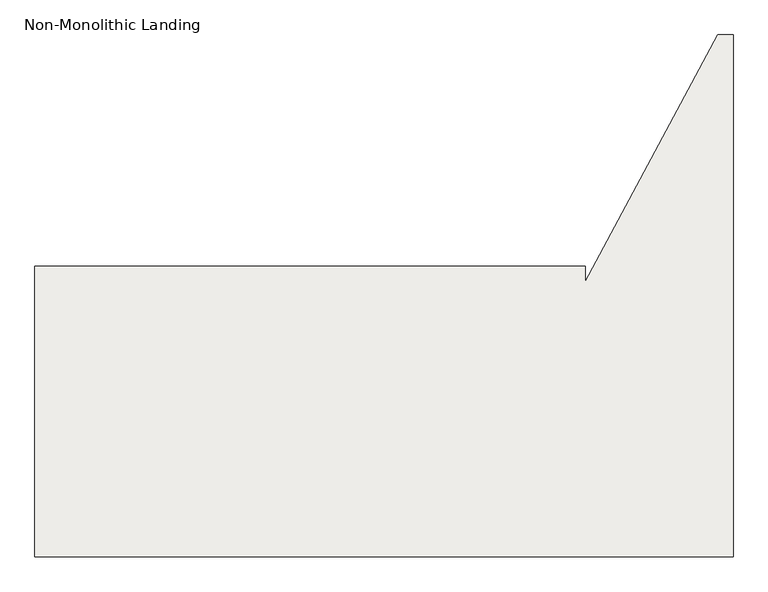
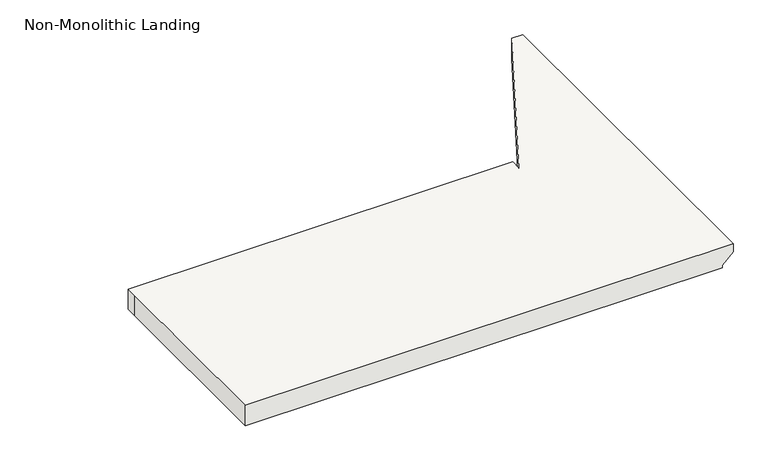
"""IFC4 building model written with IfcOpenShell, lengths in millimetres: slab geometry, Non-Monolithic Landing."""

from ifc_helpers import new_model, si_unit, origin, place, context, project, spatial, faceted_brep, source, transform, mapped, element, save


def non_monolithic_landing_7e22f3b9(model_context):
    return source(origin(), model_context, "Body", "Brep", [
        faceted_brep([(-13776.0822797, 5254.1625376, 2032.0), (-13776.0822797, 5254.1625376, 2012.95), (-13801.4822797, 5254.1625376, 1987.55), (-13801.4822797, 5254.1625376, 2032.0), (-13776.0822797, 4386.9500793, 2032.0), (-13776.0822797, 4386.9500793, 2012.95), (-13801.4822797, 4386.9500793, 1987.55), (-14022.18283, 4844.1500793, 2032.0), (-14022.18283, 4869.5500793, 2032.0), (-14936.58283, 4869.5500793, 2032.0), (-14936.58283, 4844.1500793, 2032.0), (-14936.58283, 4386.9500793, 2032.0), (-13801.4822797, 5254.1625376, 1981.2), (-13801.4822797, 4386.9500793, 1981.2), (-14936.58283, 4386.9500793, 1981.2), (-14936.58283, 4844.1500793, 1981.2), (-14936.58283, 4869.5500793, 1981.2), (-14022.18283, 4869.5500793, 1981.2), (-14022.18283, 4844.1500793, 1981.2)], [[[0, 1, 2, 3]], [[1, 0, 4, 5]], [[2, 1, 5, 6]], [[3, 7, 8, 9, 10, 11, 4, 0]], [[12, 13, 14, 15, 16, 17, 18]], [[13, 12, 2, 6]], [[7, 3, 2, 12, 18]], [[8, 7, 18, 17]], [[9, 8, 17, 16]], [[10, 9, 16, 15]], [[11, 10, 15, 14]], [[4, 11, 14, 13, 6, 5]]]),
    ])


if __name__ == "__main__":
    model = new_model("IFC4")
    model_context = context("Model", 3, world=origin())
    ifc_project = project(units=[si_unit("LENGTHUNIT", "METRE", prefix="MILLI")], contexts=[model_context])
    site = spatial("IfcSite", under=ifc_project)
    building = spatial("IfcBuilding", under=site)
    placement = place(None, origin())
    non_monolithic_landing_shape = non_monolithic_landing_7e22f3b9(model_context)
    element("IfcSlab", 1, ObjectType="Non-Monolithic Landing", at=placement, inside=building, context=model_context, shape_type="MappedRepresentation", body=[
        mapped(non_monolithic_landing_shape, transform((0.0, 0.0, 0.0), x_axis=(1.0, 0.0, 0.0), y_axis=(0.0, 1.0, 0.0), z_axis=(0.0, 0.0, 1.0))),
    ])
    save(model, "model.ifc")
